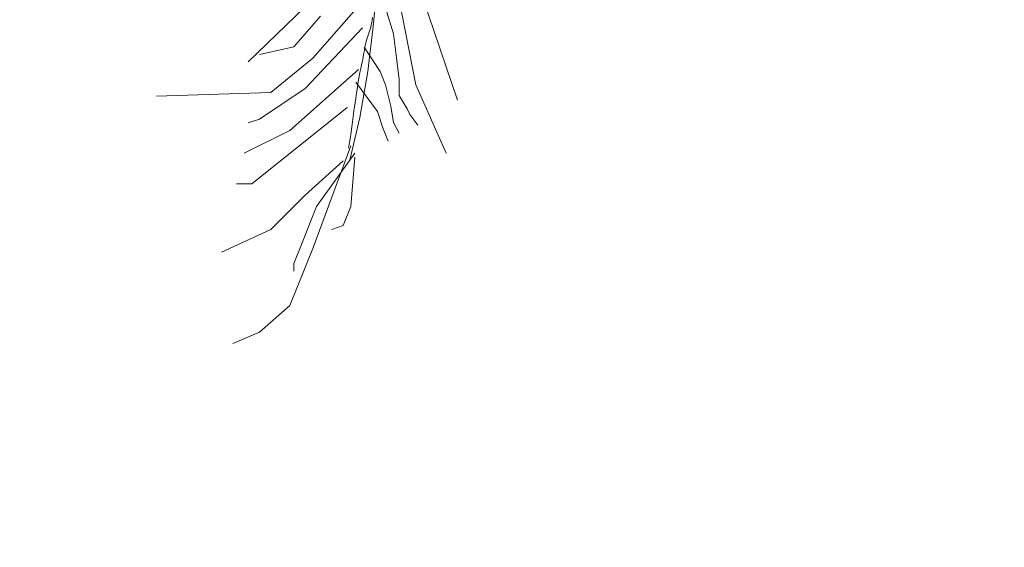
# Model space of a CAD drawing. Units: millimetres. Extents: x 595116 to 630915, y 909473 to 920225.
# Tile 68 of 134: x 629629.07 to 629636.468, y 919266.512 to 919270.478. Entities that reach past the tile are written whole.
import ezdxf

# ---------------------------------------------------------------- set-up
doc = ezdxf.new("R2010")
doc.units = ezdxf.units.MM
doc.layers.add('Dimension', color=3, linetype='Continuous', lineweight=18)
doc.layers.add('L-PLNT', color=85, linetype='Continuous', lineweight=13)
doc.styles.get("Standard").update_dxf_attribs({"font": 'arial.ttf'})
doc.dimstyles.new('ISO-25', dxfattribs={"dimtxt": 9, "dimasz": 6, "dimexe": 1.25, "dimexo": 0.625, "dimtad": 1, "dimlunit": 4, "dimtxsty": 'Standard', "dimcen": 2.5, "dimadec": 0, "dimazin": 0, "dimtfac": 1, "dimtmove": 0, "dimatfit": 3, "dimfxl": 1, "dimarcsym": 0})

# ---------------------------------------------------------------- blocks, each defined once
blk = doc.blocks.new('A$C4FB75ABC')
for p, q in [((3.386, 0.8461), (3.508, 0.4878)), ((3.3326, 0.8003), (3.0886, 0.5641)), ((3.3708, 0.7927), (3.4242, 0.5183)), ((3.3484, 0.7387), (3.34, 0.641)), ((3.325, 0.6936), (3.2182, 0.5717)), ((3.3586, 0.6905), (3.3801, 0.6206)), ((3.2335, 0.6555), (3.1801, 0.5945)), ((3.338, 0.6533), (3.3372, 0.6481)), ((3.3174, 0.6327), (3.203, 0.5107)), ((3.34, 0.641), (3.3282, 0.5451)), ((3.3341, 0.634), (3.3329, 0.6297)), ((3.3353, 0.6385), (3.3341, 0.634)), ((3.3363, 0.6432), (3.3353, 0.6385)), ((3.3372, 0.6481), (3.3363, 0.6432)), ((3.3276, 0.6135), (3.3264, 0.6095)), ((3.3289, 0.6175), (3.3276, 0.6135)), ((3.3303, 0.6215), (3.3289, 0.6175)), ((3.3316, 0.6256), (3.3303, 0.6215)), ((3.3329, 0.6297), (3.3316, 0.6256)), ((3.3801, 0.6206), (3.3855, 0.5721)), ((3.1801, 0.5945), (3.1115, 0.5793)), ((3.3209, 0.5936), (3.3532, 0.5452)), ((3.3225, 0.593), (3.3216, 0.5886)), ((3.3233, 0.5973), (3.3225, 0.593)), ((3.3242, 0.6014), (3.3233, 0.5973)), ((3.3252, 0.6055), (3.3242, 0.6014)), ((3.3264, 0.6095), (3.3252, 0.6055)), ((3.2182, 0.5717), (3.1344, 0.5031)), ((3.3191, 0.5742), (3.3181, 0.5689)), ((3.32, 0.5792), (3.3191, 0.5742)), ((3.3208, 0.584), (3.32, 0.5792)), ((3.3216, 0.5886), (3.3208, 0.584)), ((3.3855, 0.5721), (3.3909, 0.5291)), ((3.3156, 0.5574), (3.3142, 0.5507)), ((3.3169, 0.5634), (3.3156, 0.5574)), ((3.3181, 0.5689), (3.3169, 0.5634)), ((3.3098, 0.5488), (3.1725, 0.4269)), ((3.3111, 0.5347), (3.3093, 0.5249)), ((3.3127, 0.5432), (3.3111, 0.5347)), ((3.3282, 0.5451), (3.3124, 0.4531)), ((3.3142, 0.5507), (3.3127, 0.5432)), ((3.3532, 0.5452), (3.364, 0.5183)), ((3.3047, 0.5237), (3.3478, 0.4645)), ((3.3075, 0.5137), (3.3055, 0.5008)), ((3.3093, 0.5249), (3.3075, 0.5137)), ((3.364, 0.5183), (3.3747, 0.4753)), ((3.3909, 0.5291), (3.3909, 0.4968)), ((3.4242, 0.5183), (3.4852, 0.3811)), ((3.1344, 0.5031), (2.9056, 0.4955)), ((3.203, 0.5107), (3.1115, 0.4497)), ((3.3055, 0.5008), (3.3034, 0.4863)), ((3.3909, 0.4968), (3.407, 0.4699)), ((3.3034, 0.4863), (3.3013, 0.4707)), ((3.3747, 0.4753), (3.3801, 0.443)), ((3.2869, 0.4726), (3.0962, 0.3201)), ((3.2992, 0.4546), (3.297, 0.4387)), ((3.3013, 0.4707), (3.2992, 0.4546)), ((3.3478, 0.4645), (3.3586, 0.4322)), ((3.407, 0.4699), (3.4124, 0.4591)), ((3.4124, 0.4591), (3.4286, 0.4376)), ((3.1115, 0.4497), (3.0886, 0.4421)), ((3.3124, 0.4531), (3.2923, 0.3674)), ((3.297, 0.4387), (3.2949, 0.4237)), ((3.3801, 0.443), (3.3909, 0.4214)), ((3.1725, 0.4269), (3.081, 0.3811)), ((3.2949, 0.4237), (3.2929, 0.4103)), ((3.3586, 0.4322), (3.3693, 0.4053)), ((3.2945, 0.3964), (3.2182, 0.1906)), ((3.2911, 0.3992), (3.2894, 0.3911)), ((3.2929, 0.4103), (3.2911, 0.3992)), ((3.3021, 0.3811), (3.2259, 0.2744)), ((3.2793, 0.3659), (3.203, 0.2973)), ((3.3021, 0.3735), (3.2945, 0.2744)), ((3.0962, 0.3201), (3.0657, 0.3201)), ((3.203, 0.2973), (3.1344, 0.2287)), ((3.2259, 0.2744), (3.1954, 0.1982)), ((3.2945, 0.2744), (3.2793, 0.2363)), ((3.1344, 0.2287), (3.0352, 0.1829)), ((3.2793, 0.2363), (3.2564, 0.2287)), ((3.1954, 0.1982), (3.1801, 0.1601)), ((3.2182, 0.1906), (3.1725, 0.0762)), ((3.1801, 0.1601), (3.1801, 0.1448)), ((3.1725, 0.0762), (3.1115, 0.0229)), ((3.1115, 0.0229), (3.0581, 0))]:
    blk.add_line(p, q)
blk = doc.blocks.new('*D211')
at = {"layer": 'Defpoints', "color": 0, "transparency": 16777216}
for p in [(629535.3857, 919258.6624), (629586.2273, 919258.6624), (629586.2273, 919250.9434)]:
    blk.add_point(p, dxfattribs=at)
at = {"layer": 'Dimension', "color": 0, "lineweight": -2, "transparency": 16777216}
for p, q in [((629535.3857, 919258.0374), (629535.3857, 919249.6934)), ((629586.2273, 919258.0374), (629586.2273, 919249.6934)), ((629541.3857, 919250.9434), (629580.2273, 919250.9434)), ((629586.2273, 919250.9434), (629648.699, 919250.9434))]:
    blk.add_line(p, q, dxfattribs=at)
at = {"layer": 'Dimension', "color": 0, "transparency": 16777216}
for points in [[(629541.3857, 919251.9434), (629541.3857, 919249.9434), (629535.3857, 919250.9434)], [(629580.2273, 919251.9434), (629580.2273, 919249.9434), (629586.2273, 919250.9434)]]:
    blk.add_solid(points, dxfattribs=at)
at = {"layer": 'Dimension', "color": 0, "transparency": 16777216, "insert": (629620.4631, 919256.1666), "char_height": 9, "attachment_point": 5}
blk.add_mtext('4\'-3" TYP.', dxfattribs=at)
blk = doc.blocks.new('*D216')
at = {"layer": 'Defpoints', "color": 0, "transparency": 16777216}
for p in [(629743.5408, 919411.9276), (629505.0408, 919411.8279), (629743.5408, 918832.3776)]:
    blk.add_point(p, dxfattribs=at)
at = {"layer": 'Dimension', "color": 0, "lineweight": -2, "transparency": 16777216}
for p, q in [((629743.5408, 919411.3026), (629743.5408, 918831.1276)), ((629505.0408, 919411.2029), (629505.0408, 918831.1276)), ((629511.0408, 918832.3776), (629737.5408, 918832.3776))]:
    blk.add_line(p, q, dxfattribs=at)
at = {"layer": 'Dimension', "color": 0, "transparency": 16777216}
for points in [[(629511.0408, 918833.3776), (629511.0408, 918831.3776), (629505.0408, 918832.3776)], [(629737.5408, 918833.3776), (629737.5408, 918831.3776), (629743.5408, 918832.3776)]]:
    blk.add_solid(points, dxfattribs=at)
at = {"layer": 'Dimension', "color": 0, "transparency": 16777216, "insert": (629624.2908, 918837.656), "char_height": 9, "attachment_point": 5}
blk.add_mtext('19\'-10 1/2"', dxfattribs=at)

msp = doc.modelspace()

# ---------------------------------------------------------------- block references
at = {"layer": 'L-PLNT', "xscale": 3.753413438031968, "yscale": 3.753413438031968, "zscale": 3.753413438031968}
msp.add_blockref('A$C4FB75ABC', (629619.1929, 919268.043), dxfattribs=at)

# ---------------------------------------------------------------- dimensions: what is measured, and where the dimension line sits
at = {"layer": 'Dimension'}
dim = msp.add_linear_dim(base=(629743.5408, 918832.3776), p1=(629505.0408, 919411.8279), p2=(629743.5408, 919411.9276), dimstyle='ISO-25', override={"dimdec": 1, "dimlfac": 1, "dimrnd": 0, "dimzin": 1, "dimdsep": 46, "dimlunit": 4, "dimfrac": 2}, dxfattribs=at)
dim.commit()
dim.dimension.update_dxf_attribs({"geometry": '*D216', "text_midpoint": (629624.2908, 918837.656)})
dim = msp.add_linear_dim(base=(629586.2273, 919250.9434), p1=(629535.3857, 919258.6624), p2=(629586.2273, 919258.6624), text='<> TYP.', dimstyle='ISO-25', override={"dimdec": 1, "dimlfac": 1, "dimrnd": 0, "dimzin": 1, "dimdsep": 46, "dimlunit": 4, "dimfrac": 2}, dxfattribs=at)
dim.commit()
dim.dimension.update_dxf_attribs({"geometry": '*D211', "text_midpoint": (629620.4631, 919256.1666)})

doc.saveas('drawing.dxf')
